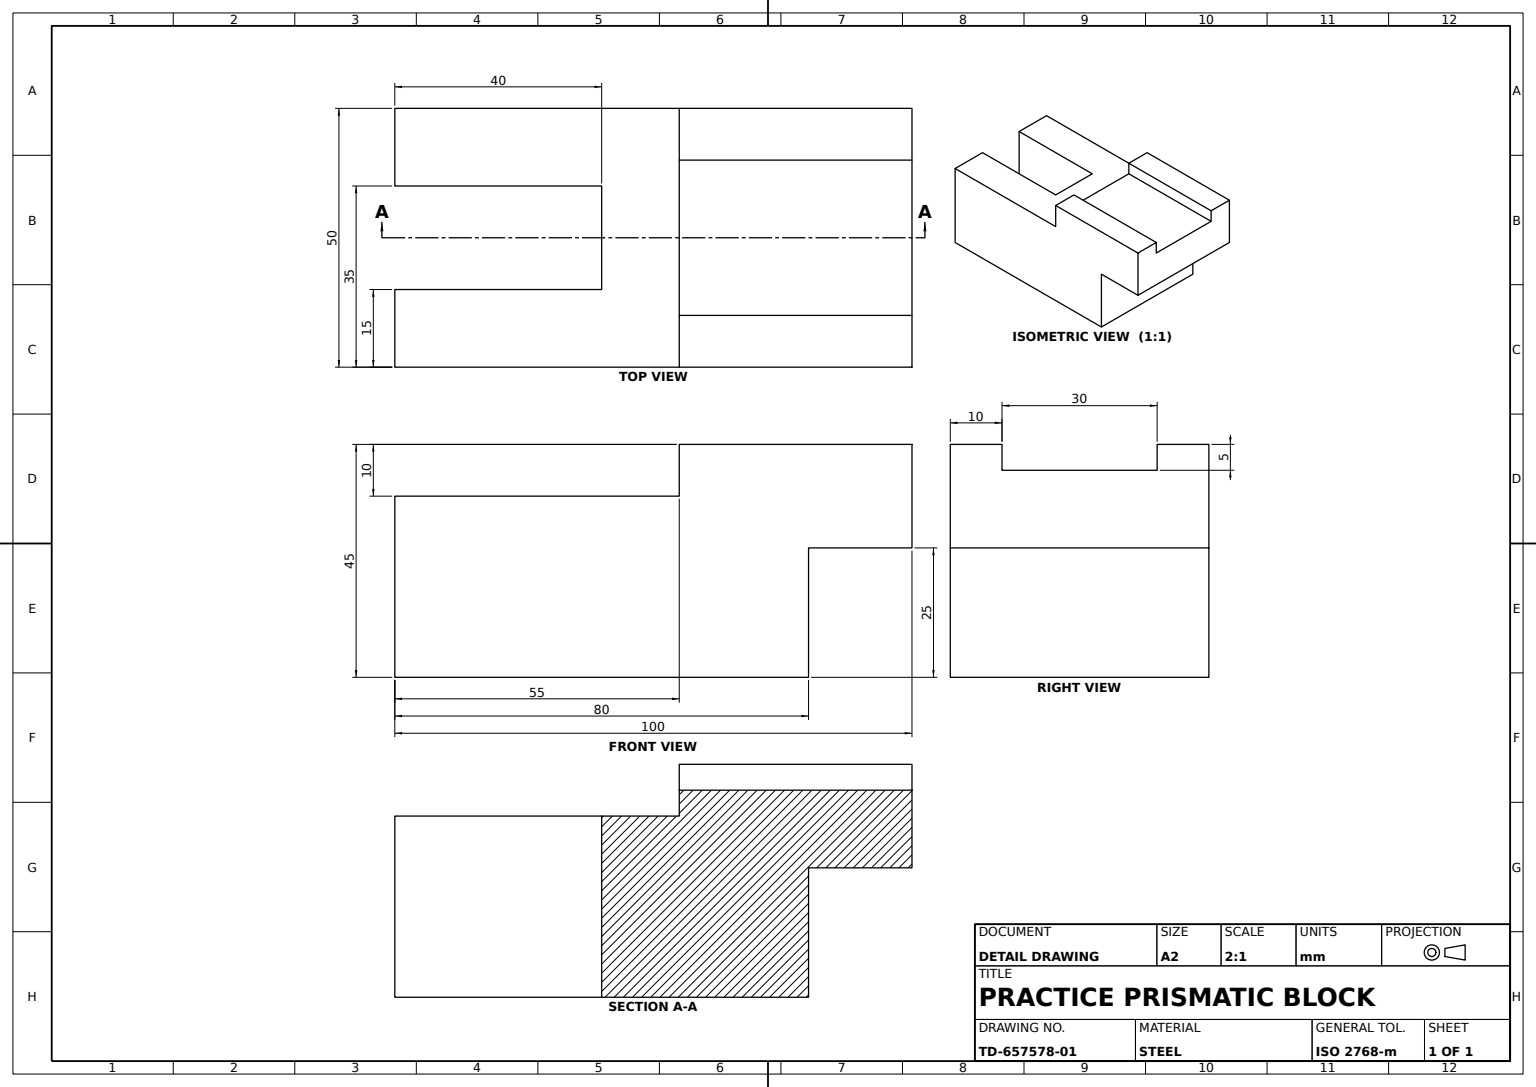
from build123d import *

# Parameters (mm, degrees)
BASE_BLOCK_DEPTH         = 50
POCKET_PROFILE_W         = 20
POCKET_PROFILE_H         = 35
RECTANGULAR_POCKET_DEPTH = 40
SLOT_PROFILE_W           = 30
SLOT_PROFILE_H           = 5
RECTANGULAR_SLOT_DEPTH   = 87.890735985


with BuildPart() as part:
    # Base Block Profile → Base Block (new body)
    with BuildSketch(Plane.XY):
        Polygon((0, 0), (80, 0), (80, 25), (100, 25), (100, 45), (55, 45), (55, 35), (0, 35), align=None)
    extrude(amount=BASE_BLOCK_DEPTH)

    # Pocket Profile → Rectangular Pocket (cut)
    with BuildSketch(Plane.ZY):
        with Locations((25, 17.5)):
            Rectangle(POCKET_PROFILE_W, POCKET_PROFILE_H)
    extrude(amount=-RECTANGULAR_POCKET_DEPTH, mode=Mode.SUBTRACT)

    # Slot Profile → Rectangular Slot (cut, through all)
    with BuildSketch(Plane.ZY.offset(-55)):
        with Locations((25, 42.5)):
            Rectangle(SLOT_PROFILE_W, SLOT_PROFILE_H)
    extrude(amount=-RECTANGULAR_SLOT_DEPTH, mode=Mode.SUBTRACT)


solid = part.part
